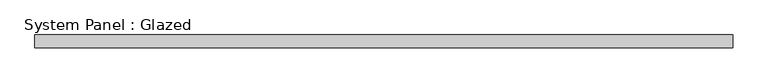
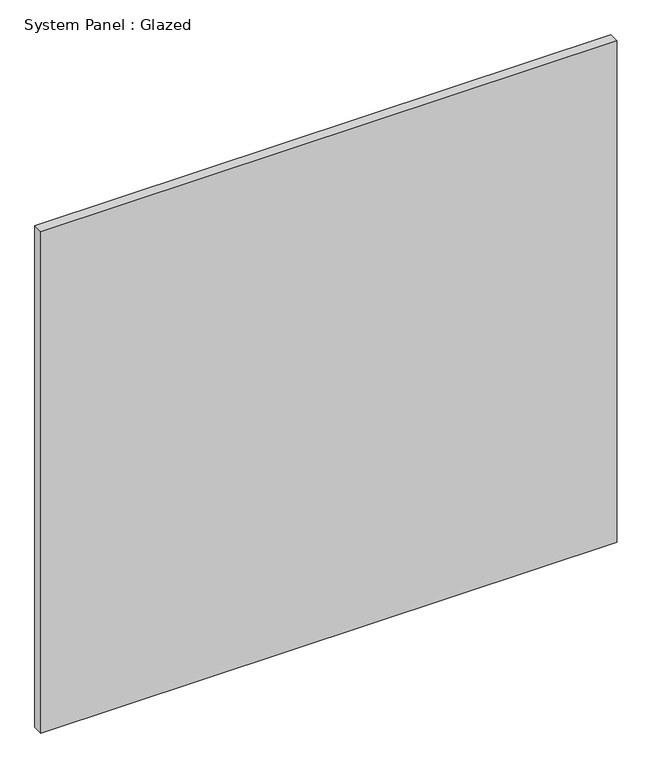
"""IFC4 building model written with IfcOpenShell, lengths in millimetres: plate geometry, System Panel : Glazed."""

from ifc_helpers import new_model, si_unit, origin, origin_with_axes, place, context, project, spatial, polyline, outline, extrude, source, transform, mapped, element, save


def system_panel_glazed_5a84bc76(model_context):
    return source(origin(), model_context, "Body", "SweptSolid", [
        extrude(outline(polyline([(695.325, 19.05), (-695.325, 19.05), (-695.325, 44.45), (695.325, 44.45), (695.325, 19.05)])), origin_with_axes(), (0.0, 0.0, 1.0), 1279.4174829),
    ])


if __name__ == "__main__":
    model = new_model("IFC4")
    model_context = context("Model", 3, world=origin())
    ifc_project = project(units=[si_unit("LENGTHUNIT", "METRE", prefix="MILLI")], contexts=[model_context])
    site = spatial("IfcSite", under=ifc_project)
    building = spatial("IfcBuilding", under=site)
    placement = place(None, origin())
    system_panel_glazed_shape = system_panel_glazed_5a84bc76(model_context)
    element("IfcPlate", 1, ObjectType="System Panel : Glazed", at=placement, inside=building, context=model_context, shape_type="MappedRepresentation", body=[
        mapped(system_panel_glazed_shape, transform((0.0, 0.0, 0.0), x_axis=(1.0, 0.0, 0.0), y_axis=(0.0, 1.0, 0.0), z_axis=(0.0, 0.0, 1.0))),
    ])
    save(model, "model.ifc")

# Revit data of these elements
# Type "System Panel : Glazed"
#   Construction Type Id = "GSP4R"
#   Analytic Construction = "1/8 in Pilkington single glazing"
#   Visual Light Transmittance = 0.9
#   Solar Heat Gain Coefficient = 0.86
#   Heat Transfer Coefficient (U) = 1.18115 BTU/(h·ft²·°F)
#   Define Thermal Properties by = 1
# Element 1 (IfcPlate, "System Panel : Glazed")
#   Materials on its faces: "Glass"
# Materials
#   "Glass": class "Glass", colour RGB 0 128 192, transparency 0.75, Description = "Soda Lime Glass", Cost = 0
